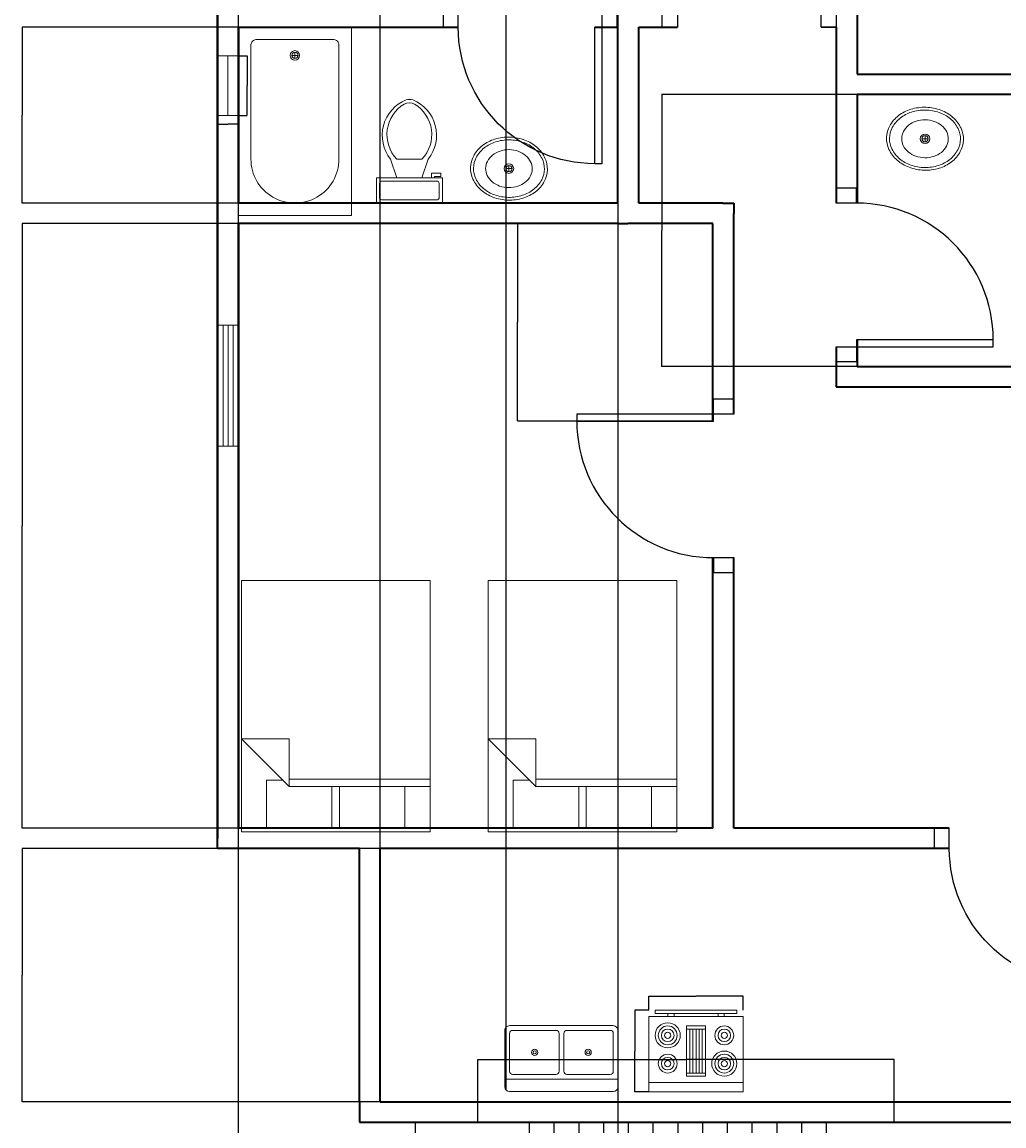
# Model space of a CAD drawing. Units: millimetres. Extents: x 31 to 27050, y -916 to 32407.
# Tile 5 of 7: x 31 to 7965, y 16782 to 25704. Entities that reach past the tile are written whole.
import ezdxf

# ---------------------------------------------------------------- set-up
doc = ezdxf.new("R2010")
doc.units = ezdxf.units.MM
for name, color, linetype, lineweight in [('A-ANNO-DIMS', 2, 'Continuous', 18), ('A-DOOR', 3, 'Continuous', 25), ('A-EQPM', 8, 'Continuous', 18), ('A-FLOR-FIXT', 9, 'Continuous', 18), ('A-FLOR-STRS', 7, 'Continuous', 25), ('A-FURN', 8, 'Continuous', 13), ('A-GLAZ', 4, 'Continuous', 18), ('A-WALL', 7, 'Continuous', 35)]:
    doc.layers.add(name, color=color, linetype=linetype, lineweight=lineweight)
doc.styles.get("Standard").update_dxf_attribs({"font": 'arial.ttf'})
doc.dimstyles.get("Standard").update_dxf_attribs({"dimtxt": 0.18, "dimasz": 0.18, "dimexe": 0.18, "dimexo": 0.0625, "dimgap": 0.09, "dimtad": 0, "dimtih": 1, "dimtoh": 1, "dimdec": 4, "dimzin": 0, "dimdsep": 46, "dimtxsty": 'Standard', "dimcen": 0.09, "dimadec": 0, "dimazin": 0, "dimtfac": 1, "dimtdec": 4, "dimtofl": 0, "dimtmove": 0, "dimatfit": 3, "dimfxl": 1, "dimtolj": 1, "dimtzin": 0, "dimarcsym": 0})

# ---------------------------------------------------------------- blocks, each defined once
blk = doc.blocks.new('Range-Oven - 30 in top')
for p, q in [((0, -3), (30, -3)), ((12, -6), (18, -6)), ((13, -19.999996), (13, -6)), ((14, -6), (14, -19.999996)), ((15, -19.999996), (15, -6)), ((16, -6), (16, -19.999996)), ((17, -19.999996), (17, -6)), ((18, -19.999996), (12, -19.999996)), ((6.000000000000003, -23.99999600000001), (6.000000000000003, -24.999996)), ((8.000000000000004, -24.999996), (8.000000000000004, -23.99999600000001)), ((22.00000000000001, -24.999996), (22.00000000000001, -23.99999600000001)), ((24, -23.99999600000001), (24, -24.999996))]:
    blk.add_line(p, q)
for points in [[(0, -23.99999600000001), (0, 0), (30, 0), (30, -23.99999600000001)], [(12, -20.999996), (12, -5), (18, -5), (18, -20.999996)], [(2.000000000000003, -25.999996), (2.000000000000003, -24.999996), (28.00000000000001, -24.999996), (28.00000000000001, -25.999996)]]:
    blk.add_lwpolyline(points, close=True)
for centre, radius in [((6.000000000000003, -9.0000002), 4), ((6.000000000000003, -9.0000002), 3), ((6.000000000000003, -9.0000002), 2), ((24, -9.0000002), 3), ((24, -9.0000002), 2), ((6.000000000000003, -9.0000002), 1), ((24, -9.0000002), 1), ((24, -18), 4), ((6.000000000000003, -18), 3), ((6.000000000000003, -18), 2), ((6.000000000000003, -18), 1), ((24, -18), 3), ((24, -18), 2), ((24, -18), 1)]:
    blk.add_circle(centre, radius)
blk = doc.blocks.new('Sink-double - 36 in top')
for p, q in [((-18, -4), (18, -4)), ((-0.75, -18.5), (-0.75, -6.5)), ((0.75, -6.5), (0.75, -18.5))]:
    blk.add_line(p, q)
for points in [[(-16.5, 0), (16.5, 0)], [(-18, -19.5), (-18, -1.5)], [(18, -1.5), (18, -19.5)], [(-16.5, -18.5), (-16.5, -6.5)], [(-15.5, -5.5), (-1.75, -5.5)], [(1.75, -5.5), (15.5, -5.5)], [(16.5, -6.5), (16.5, -18.5)], [(16.5, -21), (-16.5, -21)], [(-1.75, -19.5), (-15.5, -19.5)], [(15.5, -19.5), (1.75, -19.5)]]:
    blk.add_lwpolyline(points)
for centre, radius in [((-8.5, -12.5), 1), ((-8.5, -12.5), 0.5), ((8.5, -12.5), 1), ((8.5, -12.5), 0.5)]:
    blk.add_circle(centre, radius)
for centre, radius, start, end in [((-16.5, -1.5), 1.5, 90, 180), ((16.5, -1.5), 1.5, 0, 90), ((-15.5, -6.5), 1, 90, 180), ((-1.75, -6.5), 1, 0, 90), ((1.75, -6.5), 1, 90, 180), ((15.5, -6.5), 1, 0, 90), ((-16.5, -19.5), 1.5, 180, 270), ((-15.5, -18.5), 1, 180, 270), ((-1.75, -18.5), 1, 270, 0), ((1.75, -18.5), 1, 180, 270), ((15.5, -18.5), 1, 270, 0), ((16.5, -19.5), 1.5, 270, 0)]:
    blk.add_arc(centre, radius, start, end)
blk = doc.blocks.new('Bath Tub - 26 x 60 in.')
for p, q in [((9, -17), (9, -19)), ((8, -18), (10, -18))]:
    blk.add_line(p, q)
blk.add_lwpolyline([(0, -36), (0, 0), (60, 0), (60, -36)], close=True)
for points in [[(4, -30), (4, -6)], [(6, -4), (42, -4)], [(42, -32), (6, -32)]]:
    blk.add_lwpolyline(points)
for radius in [1.5, 1]:
    blk.add_circle((9, -18), radius)
for centre, radius, start, end in [((5.75, -5.75), 1.767766999999999, 81.86989999999999, 188.1301), ((42, -18), 14, 270, 90), ((5.75, -30.25), 1.767766999999999, 171.8699, 278.1301)]:
    blk.add_arc(centre, radius, start, end)
blk = doc.blocks.new('Sink - Oval top')
for p, q in [((-1, 0), (1, 0)), ((0, 1), (0, -1))]:
    blk.add_line(p, q)
for points in [[(-12.23371880354079, 0.3941914712607968, 0.1176342565883263), (-11.46456229543957, -3.361933235489118, 0.104469279667093), (-8.878748691070427, -6.803541973650567, 0.0900157896014849), (-5.082757700676665, -9.072309807490512, 0.0819199491592185), (-0.3227280122732736, -10.01585280257211, 0.0819199491592091), (4.488169920880977, -9.380701564817912, 0.0900157896014801), (8.422342359155778, -7.36101289847943, 0.1044692796670922), (11.22435122606941, -4.093009071543406, 0.1176342565883338), (12.23371880354091, -0.3941914712607968, 0.1176342565883057), (11.46456229543992, 3.361933235488777, 0.1044692796670849), (8.878748691070427, 6.803541973650567, 0.0900157896014884), (5.082757700676324, 9.072309807490681, 0.0819199491592058), (0.3227280122732736, 10.01585280257211, 0.081919949159207), (-4.488169920880864, 9.380701564817969, 0.0900157896014802), (-8.422342359155778, 7.36101289847943, 0.1044692796670951), (-11.22435122606919, 4.093009071543633, 0.1176342565883402)], [(-11.28627986850119, 0.1590597164737346, 0.1186217001864142), (-10.51590095791209, -3.253161772358112, 0.1046781721811095), (-8.071803350560115, -6.358618019863342, 0.0895620664691738), (-4.537699193222351, -8.366971929609804, 0.0811846988912177), (-0.1289739026695997, -9.15150355811437, 0.0811846988912276), (4.300109150126218, -8.491524865184601, 0.0895620664691798), (7.889406708212618, -6.583562428127606, 0.1046781721811044), (10.42004782883111, -3.548216131892445, 0.1186217001864013), (11.28627986850119, -0.1590597164736209, 0.1186217001863945), (10.51590095791221, 3.253161772357998, 0.1046781721811069), (8.071803350560115, 6.358618019863342, 0.0895620664691756), (4.537699193222124, 8.366971929609917, 0.081184698891216), (0.1289739026695997, 9.151503558114428, 0.0811846988912142), (-4.300109150125877, 8.491524865184829, 0.0895620664691747), (-7.889406708212618, 6.583562428127606, 0.1046781721811045), (-10.42004782883111, 3.548216131892445, 0.1186217001863946)], [(-7.420452389032902, 0.0829876781601797, 0.1182825673856775), (-6.907065465214486, -2.1674649380775, 0.1046074595377274), (-5.294791470712084, -4.209988192029413, 0.0897179636260996), (-2.966599981142508, -5.528122152688069, 0.0814360825277113), (-0.0675135187855176, -6.036810076758797, 0.0814360825277218), (2.84222437824053, -5.593085960977873, 0.0897179636261315), (5.199312936802016, -4.327350491993342, 0.1046074595376878), (6.85686365682659, -2.321395784920355, 0.1182825673856714), (7.420452389033016, -0.0829876781601797, 0.1182825673856961), (6.907065465214486, 2.167464938077614, 0.1046074595377135), (5.294791470712084, 4.209988192029413, 0.0897179636261265), (2.966599981142621, 5.528122152687842, 0.0814360825277426), (0.0675135187855176, 6.036810076758797, 0.0814360825277225), (-2.842224378240644, 5.593085960977873, 0.0897179636261212), (-5.199312936802016, 4.327350491993342, 0.1046074595377049), (-6.856863656826476, 2.321395784920355, 0.1182825673856712)]]:
    blk.add_lwpolyline(points, format="xyb", close=True)
for radius in [1.5, 1]:
    blk.add_circle((0, 0), radius)
blk = doc.blocks.new('Toilet - top')
for p, q in [((9.5, -6), (9.5, -2)), ((-10, -8.5), (-8, -8.5)), ((-10, -9.5), (-10, -8.5)), ((-7, -9.5), (-10, -9.5)), ((-8, -8.5), (-8, -8)), ((-7, -8), (-7, -9.5)), ((-4, -8), (-6, -14)), ((4, -8), (6, -14)), ((4, -14), (-4, -14))]:
    blk.add_line(p, q)
blk.add_lwpolyline([(10.5, -8), (10.5, 0), (-10.5, 0), (-10.5, -8)], close=True)
for points in [[(-9.5, -2), (-9.5, -6)], [(8.5, -1), (-8.5, -1)], [(-8.5, -7), (8.5, -7)]]:
    blk.add_lwpolyline(points)
for centre, radius, start, end in [((-8.625, -1.875), 0.8838834999999999, 81.86989999999999, 188.1301), ((8.625, -1.875), 0.8838834999999999, 351.8699, 98.13009999999998), ((-8.625, -6.125), 0.8838834999999999, 171.869898, 278.1301), ((8.625, -6.125), 0.8838834999999999, 261.8699, 8.130099999999993), ((3.519562435188956, -21.58049502388982), 12.16902005083646, 141.4691096810948, 247.9714346835576), ((4.199957580658807, -21.81740929088453), 11.3291791325804, 136.3677254423718, 238.946823937405), ((-3.519499936778316, -21.58047137067522), 12.16903423757823, 292.0284332733152, 38.53070636800453), ((-4.199890672038477, -21.81738596564128), 11.32918622148567, 301.0530065773863, 43.63209216694732), ((2.09660981727e-05, -27.87646475467881), 4, 245.7318247449371, 294.2681740488959), ((2.09415214183e-05, -28.99996806116075), 4, 254.8605283244437, 285.1394707718433)]:
    blk.add_arc(centre, radius, start, end)
blk = doc.blocks.new('Bed - Queen')
for p, q in [((0, -80.00003000000002), (0, 0)), ((0, 0), (59.99998999999999, 0)), ((59.99998999999999, 0), (59.99998999999999, -80.00003000000002)), ((7.99999, -1.200000000000017), (28.79998, -1.200000000000017)), ((7.99999, -14.4), (7.99999, -1.200000000000017)), ((28.79998, -1.200000000000017), (28.79998, -14.4)), ((31.19999, -1.200000000000017), (51.99999000000001, -1.200000000000017)), ((31.19999, -14.4), (31.19999, -1.200000000000017)), ((51.99999000000001, -1.200000000000017), (51.99999000000001, -16.4)), ((0, -14.4), (44.79999999999999, -14.4)), ((44.79999999999999, -16.80000000000001), (0, -16.80000000000001)), ((59.99998999999999, -29.60000000000001), (44.79999999999999, -14.4)), ((44.79999999999999, -14.4), (44.79999999999999, -29.60000000000001)), ((51.99999000000001, -16.4), (46.79936, -16.4)), ((44.79999999999999, -29.60000000000001), (59.99998999999999, -29.60000000000001)), ((59.99998999999999, -80.00003000000002), (0, -80.00003000000002))]:
    blk.add_line(p, q)
blk = doc.blocks.new('Window - Wood Frame 36 in. Wide plan')
for p, q in [((0, 6), (0, 0)), ((0, 4.5), (36, 4.5)), ((36, 6), (36, 0)), ((0, 3), (36, 3)), ((0, 1.5), (36, 1.5))]:
    blk.add_line(p, q)
blk = doc.blocks.new('DOOR-SINGLE-1104')
for p, q in [((56.41678681898429, 1104.337341461596), (-7.18501e-11, 1104.337341461596)), ((-7.18501e-11, 1104.337341461596), (-7.18501e-11, 3.638e-12)), ((56.41678681898429, 7.276e-12), (56.41678681898429, 1104.337341461596)), ((-1226.913698425656, -163.8831223050438), (-1226.913698425656, 3.638e-12)), ((-1104.337341461589, 3.638e-12), (-1226.913698425656, 7.276e-12)), ((-1104.337341461589, 3.638e-12), (-1104.337341461589, -163.8831223050438)), ((-7.18501e-11, 3.638e-12), (56.41678681898429, 7.276e-12)), ((56.41678681898429, -163.8831223050438), (56.41678681898429, 3.638e-12)), ((56.41678681898429, 3.638e-12), (178.9931437830519, 3.638e-12)), ((178.9931437830519, 3.638e-12), (178.9931437830519, -163.8831223050438)), ((-1104.337341461589, -163.8831223050438), (-1226.913698425656, -163.8831223050438)), ((178.9931437830519, -163.8831223050438), (56.41678681898429, -163.8831223050438))]:
    blk.add_line(p, q)
blk.add_arc((0, 3.638e-12), 1104.337341461589, 90, 180)
blk = doc.blocks.new('STAIR-RETURN-2400')
for p, q in [((9.095e-13, 2345.636859649549), (9.095e-13, -1.819e-12)), ((200.0000000000009, 2345.636859649549), (200.0000000000009, -1.819e-12)), ((400.0000000000008, 2345.636859649549), (400.0000000000008, -1.819e-12)), ((600.0000000000008, 2345.636859649549), (600.0000000000008, -1.819e-12)), ((800.0000000000008, 2345.636859649552), (800.0000000000008, 1.819e-12)), ((1000.000000000001, 2345.636859649556), (1000.000000000001, 5.457e-12)), ((1200.000000000001, 2345.636859649556), (1200.000000000001, 5.457e-12)), ((1400.000000000001, 2345.636859649556), (1400.000000000001, 5.457e-12)), ((1600.000000000001, 2345.636859649559), (1600.000000000001, 9.0949e-12)), ((1800.000000000001, 2345.636859649559), (1800.000000000001, 9.0949e-12)), ((2000.000000000001, 2345.636859649559), (2000.000000000001, 9.0949e-12)), ((2200.000000000001, 2345.636859649563), (2200.000000000001, 1.27329e-11)), ((2400.000000000001, 2345.636859649563), (2400.000000000001, 1.27329e-11)), ((-415.9249645337103, 697.4958917418807), (-415.9249645337103, 1817.654410237617)), ((-415.9249645337103, 1817.654410237617), (2588.331988211024, 1817.654410237617)), ((9.095e-13, 1172.818429824772), (9.095e-13, 1272.818429824772)), ((9.095e-13, 1272.818429824772), (2400.000000000001, 1272.818429824774)), ((2400.000000000001, 1272.818429824774), (2400.000000000001, 1072.818429824774)), ((2400.000000000001, 1072.818429824774), (9.095e-13, 1072.818429824774)), ((2597.09055342863, 697.4958917418807), (-415.9249645337103, 697.4958917418807))]:
    blk.add_line(p, q)
blk.add_lwpolyline([(2948.607295106225, 1817.654410237617), (2588.331988211024, 2025.65945565594), (2588.331988211024, 1609.649364819299)], close=True)
blk = doc.blocks.new('WIN-BATH-482')
for p, q in [((0, 3.638e-12), (-168.350650710694, 3.638e-12)), ((-84.17532535534633, -482.3297634273148), (-84.17532535534701, 3.638e-12)), ((-168.350650710694, -482.3297634273148), (1.3642e-12, -482.3297634273148))]:
    blk.add_line(p, q)
blk = doc.blocks.new('*D30')
at = {"layer": 'A-ANNO-DIMS', "color": 0, "lineweight": -2, "transparency": 16777216}
for p, q in [((5095.835211668338, 17717.30289499948), (5095.835211668338, 17831.72039499948)), ((5096.015211668339, 17831.54039499948), (5475.759816033958, 17831.54039499948)), ((5857.655211668338, 17831.54039499948), (5477.910607302717, 17831.54039499948)), ((5857.835211668338, 17717.30289499948), (5857.835211668338, 17831.72039499948))]:
    blk.add_line(p, q, dxfattribs=at)
at = {"layer": 'A-ANNO-DIMS', "color": 0, "transparency": 16777216}
for points in [[(5096.015211668339, 17831.57039499948), (5096.015211668339, 17831.51039499948), (5095.835211668338, 17831.54039499948)], [(5857.655211668338, 17831.57039499948), (5857.655211668338, 17831.51039499948), (5857.835211668338, 17831.54039499948)]]:
    blk.add_solid(points, dxfattribs=at)
at = {"layer": 'Defpoints', "color": 0, "transparency": 16777216}
for p in [(5095.835211668338, 17831.54039499948), (5095.835211668338, 17717.24039499948), (5857.835211668338, 17717.24039499948)]:
    blk.add_point(p, dxfattribs=at)
at = {"layer": 'A-ANNO-DIMS', "color": 0, "transparency": 16777216, "insert": (5476.835211668338, 17831.54039499948), "char_height": 0.18, "attachment_point": 5}
blk.add_mtext('\\A1;RANGE 762 TYP.', dxfattribs=at)
blk = doc.blocks.new('*D31')
at = {"layer": 'A-ANNO-DIMS', "color": 0, "lineweight": -2, "transparency": 16777216}
for p, q in [((5095.77271166834, 17717.24039499949), (4981.355211668341, 17717.24039499949)), ((4981.535211668341, 17717.06039499949), (4981.535211668341, 17387.22234893728)), ((4981.535211668341, 17057.02049659949), (4981.535211668341, 17386.8585426617)), ((5095.77271166834, 17056.84049659949), (4981.355211668341, 17056.84049659949))]:
    blk.add_line(p, q, dxfattribs=at)
at = {"layer": 'A-ANNO-DIMS', "color": 0, "transparency": 16777216}
for points in [[(4981.505211668341, 17717.06039499949), (4981.565211668342, 17717.06039499949), (4981.535211668341, 17717.24039499949)], [(4981.505211668341, 17057.02049659949), (4981.565211668342, 17057.02049659949), (4981.535211668341, 17056.84049659949)]]:
    blk.add_solid(points, dxfattribs=at)
at = {"layer": 'Defpoints', "color": 0, "transparency": 16777216}
for p in [(5095.83521166834, 17717.24039499949), (4981.535211668341, 17056.84049659949), (5095.83521166834, 17056.84049659949)]:
    blk.add_point(p, dxfattribs=at)
at = {"layer": 'A-ANNO-DIMS', "color": 0, "transparency": 16777216, "insert": (4981.535211668346, 17387.04044579948), "char_height": 0.18, "attachment_point": 5}
blk.add_mtext('\\A1;660 TYP.', dxfattribs=at)
blk = doc.blocks.new('*D40')
at = {"layer": 'A-ANNO-DIMS', "color": 0, "lineweight": -2, "transparency": 16777216}
for p, q in [((3712.669091999182, 16813.12429635636), (3712.669091999182, 17317.92163530235)), ((3712.849091999181, 17317.74163530235), (5393.307977617239, 17317.74163530235)), ((7077.021351639117, 17317.74163530235), (5396.562466021059, 17317.74163530235)), ((7077.201351639117, 16813.12429635636), (7077.201351639117, 17317.92163530235))]:
    blk.add_line(p, q, dxfattribs=at)
at = {"layer": 'A-ANNO-DIMS', "color": 0, "transparency": 16777216}
for points in [[(3712.849091999181, 17317.77163530235), (3712.849091999181, 17317.71163530235), (3712.669091999182, 17317.74163530235)], [(7077.021351639117, 17317.77163530235), (7077.021351639117, 17317.71163530235), (7077.201351639117, 17317.74163530235)]]:
    blk.add_solid(points, dxfattribs=at)
at = {"layer": 'Defpoints', "color": 0, "transparency": 16777216}
for p in [(7077.201351639117, 17317.74163530235), (3712.669091999182, 16813.06179635636), (7077.201351639117, 16813.06179635636)]:
    blk.add_point(p, dxfattribs=at)
at = {"layer": 'A-ANNO-DIMS', "color": 0, "transparency": 16777216, "insert": (5394.935221819149, 17317.74163530235), "char_height": 0.18, "attachment_point": 5}
blk.add_mtext('\\A1;RETURN STAIR 3365 TYP.', dxfattribs=at)
blk = doc.blocks.new('*D41')
at = {"layer": 'A-ANNO-DIMS', "color": 0, "lineweight": -2, "transparency": 16777216}
for p, q in [((3712.606591999184, 16813.06179635637), (3207.809253053195, 16813.06179635637)), ((3207.989253053195, 16812.88179635637), (3207.989253053195, 15640.42533106092)), ((3207.989253053195, 14467.60493670681), (3207.989253053195, 15640.06140200226)), ((3712.606591999184, 14467.4249367068), (3207.809253053195, 14467.4249367068))]:
    blk.add_line(p, q, dxfattribs=at)
at = {"layer": 'A-ANNO-DIMS', "color": 0, "transparency": 16777216}
for points in [[(3207.959253053195, 16812.88179635637), (3208.019253053195, 16812.88179635637), (3207.989253053195, 16813.06179635637)], [(3207.959253053195, 14467.60493670681), (3208.019253053195, 14467.60493670681), (3207.989253053195, 14467.4249367068)]]:
    blk.add_solid(points, dxfattribs=at)
at = {"layer": 'Defpoints', "color": 0, "transparency": 16777216}
for p in [(3207.989253053195, 16813.06179635637), (3712.669091999184, 16813.06179635637), (3712.669091999184, 14467.4249367068)]:
    blk.add_point(p, dxfattribs=at)
at = {"layer": 'A-ANNO-DIMS', "color": 0, "transparency": 16777216, "insert": (3207.989253053199, 15640.24336653158), "char_height": 0.18, "attachment_point": 5}
blk.add_mtext('\\A1;2346 TYP.', dxfattribs=at)
blk = doc.blocks.new('*D44')
at = {"layer": 'A-ANNO-DIMS', "color": 0, "lineweight": -2, "transparency": 16777216}
for p, q in [((1778.435147825163, 25432.43652884754), (1850.902112339262, 25432.43652884754)), ((1850.722112339262, 25432.25652884754), (1850.722112339262, 25191.4547781025)), ((1850.722112339262, 24950.28676542022), (1850.722112339262, 25191.08851616526)), ((1778.435147825163, 24950.10676542022), (1850.902112339262, 24950.10676542022))]:
    blk.add_line(p, q, dxfattribs=at)
at = {"layer": 'A-ANNO-DIMS', "color": 0, "transparency": 16777216}
for points in [[(1850.692112339262, 25432.25652884754), (1850.752112339262, 25432.25652884754), (1850.722112339262, 25432.43652884754)], [(1850.692112339262, 24950.28676542022), (1850.752112339262, 24950.28676542022), (1850.722112339262, 24950.10676542022)]]:
    blk.add_solid(points, dxfattribs=at)
at = {"layer": 'Defpoints', "color": 0, "transparency": 16777216}
for p in [(1778.372647825163, 25432.43652884754), (1850.722112339262, 25432.43652884754), (1778.372647825163, 24950.10676542022)]:
    blk.add_point(p, dxfattribs=at)
at = {"layer": 'A-ANNO-DIMS', "color": 0, "transparency": 16777216, "insert": (1850.722112339269, 25191.27164713387), "char_height": 0.18, "attachment_point": 5}
blk.add_mtext('\\A1;BATH WINDOW 482 TYP.', dxfattribs=at)
blk = doc.blocks.new('*D45')
at = {"layer": 'A-ANNO-DIMS', "color": 0, "lineweight": -2, "transparency": 16777216}
for p, q in [((1610.021997114467, 24950.04426542021), (1610.021997114467, 24877.57730090611)), ((1778.372647825162, 24950.04426542021), (1778.372647825162, 24877.57730090611)), ((1610.201997114467, 24877.75730090611), (1693.607779495735, 24877.75730090611)), ((1778.192647825162, 24877.75730090611), (1694.786865443894, 24877.75730090611))]:
    blk.add_line(p, q, dxfattribs=at)
at = {"layer": 'A-ANNO-DIMS', "color": 0, "transparency": 16777216}
for points in [[(1610.201997114467, 24877.78730090611), (1610.201997114467, 24877.72730090611), (1610.021997114467, 24877.75730090611)], [(1778.192647825162, 24877.78730090611), (1778.192647825162, 24877.72730090611), (1778.372647825162, 24877.75730090611)]]:
    blk.add_solid(points, dxfattribs=at)
at = {"layer": 'Defpoints', "color": 0, "transparency": 16777216}
for p in [(1610.021997114467, 24950.10676542021), (1778.372647825162, 24950.10676542021), (1778.372647825162, 24877.75730090611)]:
    blk.add_point(p, dxfattribs=at)
at = {"layer": 'A-ANNO-DIMS', "color": 0, "transparency": 16777216, "insert": (1694.197322469815, 24877.75730090611), "char_height": 0.18, "attachment_point": 5}
blk.add_mtext('\\A1;168 TYP.', dxfattribs=at)
blk = doc.blocks.new('*D53')
at = {"layer": 'A-ANNO-DIMS', "color": 0, "lineweight": -2, "transparency": 16777216}
for p, q in [((1778.310148000001, 25663.64813600002), (30.84199699999976, 25663.64813600002)), ((31.02199699999987, 25663.46813600001), (31.02199700000003, 24952.32387752935)), ((31.02199700000019, 24240.81569000001), (31.02199700000003, 24951.95994847068)), ((1778.310148000001, 24240.63569000001), (30.84199700000008, 24240.63569000001))]:
    blk.add_line(p, q, dxfattribs=at)
at = {"layer": 'A-ANNO-DIMS', "color": 0, "transparency": 16777216}
for points in [[(30.99199699999987, 25663.46813600001), (31.05199699999988, 25663.46813600001), (31.02199699999987, 25663.64813600002)], [(30.99199700000019, 24240.81569000001), (31.05199700000019, 24240.81569000001), (31.02199700000019, 24240.63569000001)]]:
    blk.add_solid(points, dxfattribs=at)
at = {"layer": 'Defpoints', "color": 0, "transparency": 16777216}
for p in [(31.02199699999987, 25663.64813600002), (1778.372648000001, 25663.64813600002), (1778.372648000001, 24240.63569000001)]:
    blk.add_point(p, dxfattribs=at)
at = {"layer": 'A-ANNO-DIMS', "color": 0, "transparency": 16777216, "insert": (31.02199700000709, 24952.14191300001), "char_height": 0.18, "attachment_point": 5}
blk.add_mtext('\\A1;1423', dxfattribs=at)
blk = doc.blocks.new('*D54')
at = {"layer": 'A-ANNO-DIMS', "color": 0, "lineweight": -2, "transparency": 16777216}
for p, q in [((1778.310148000001, 24076.75256800001), (30.84199699999943, 24076.75256800001)), ((31.02199699999948, 24076.57256800001), (31.02199700000003, 21633.2176101378)), ((31.02199700000057, 19189.498846), (31.02199700000003, 21632.85380386222)), ((1778.310148000001, 19189.318846), (30.84199700000052, 19189.318846))]:
    blk.add_line(p, q, dxfattribs=at)
at = {"layer": 'A-ANNO-DIMS', "color": 0, "transparency": 16777216}
for points in [[(30.99199699999948, 24076.57256800001), (31.05199699999948, 24076.57256800001), (31.02199699999948, 24076.75256800001)], [(30.99199700000057, 19189.498846), (31.05199700000057, 19189.498846), (31.02199700000057, 19189.318846)]]:
    blk.add_solid(points, dxfattribs=at)
at = {"layer": 'Defpoints', "color": 0, "transparency": 16777216}
for p in [(31.02199699999948, 24076.75256800001), (1778.372648000001, 24076.75256800001), (1778.372648000001, 19189.318846)]:
    blk.add_point(p, dxfattribs=at)
at = {"layer": 'A-ANNO-DIMS', "color": 0, "transparency": 16777216, "insert": (31.02199700000615, 21633.03570700001), "char_height": 0.18, "attachment_point": 5}
blk.add_mtext('\\A1;4887', dxfattribs=at)
blk = doc.blocks.new('*D55')
at = {"layer": 'A-ANNO-DIMS', "color": 0, "lineweight": -2, "transparency": 16777216}
for p, q in [((2925.628986000001, 19025.43572400001), (30.84199699999987, 19025.43572400001)), ((31.0219969999998, 19025.255724), (31.02199700000003, 18001.3722246378)), ((31.02199700000026, 16977.12491900001), (31.02199700000003, 18001.00841836222)), ((2925.628986000001, 16976.94491900001), (30.84199700000032, 16976.94491900001))]:
    blk.add_line(p, q, dxfattribs=at)
at = {"layer": 'A-ANNO-DIMS', "color": 0, "transparency": 16777216}
for points in [[(30.9919969999998, 19025.255724), (31.0519969999998, 19025.255724), (31.0219969999998, 19025.43572400001)], [(30.99199700000025, 16977.12491900001), (31.05199700000026, 16977.12491900001), (31.02199700000026, 16976.94491900001)]]:
    blk.add_solid(points, dxfattribs=at)
at = {"layer": 'Defpoints', "color": 0, "transparency": 16777216}
for p in [(31.0219969999998, 19025.43572400001), (2925.691486000001, 19025.43572400001), (2925.691486000001, 16976.94491900001)]:
    blk.add_point(p, dxfattribs=at)
at = {"layer": 'A-ANNO-DIMS', "color": 0, "transparency": 16777216, "insert": (31.02199700000512, 18001.1903215), "char_height": 0.18, "attachment_point": 5}
blk.add_mtext('\\A1;2048.5', dxfattribs=at)
blk = doc.blocks.new('*D61')
at = {"layer": 'A-ANNO-DIMS', "color": 0, "lineweight": -2, "transparency": 16777216}
for p, q in [((1778.372648, 7250.606205), (1778.372648000001, 32406.711259)), ((1778.552648000001, 32406.531259), (3312.109331318556, 32406.531259)), ((4846.592413000001, 32406.531259), (3313.035729681448, 32406.531259)), ((4846.772413, 7250.606205), (4846.772413000001, 32406.711259))]:
    blk.add_line(p, q, dxfattribs=at)
at = {"layer": 'A-ANNO-DIMS', "color": 0, "transparency": 16777216}
for points in [[(1778.552648000001, 32406.561259), (1778.552648000001, 32406.501259), (1778.372648000001, 32406.531259)], [(4846.592413000001, 32406.561259), (4846.592413000001, 32406.501259), (4846.772413000001, 32406.531259)]]:
    blk.add_solid(points, dxfattribs=at)
at = {"layer": 'Defpoints', "color": 0, "transparency": 16777216}
for p in [(4846.772413000001, 32406.531259), (1778.372648, 7250.543705), (4846.772413, 7250.543705)]:
    blk.add_point(p, dxfattribs=at)
at = {"layer": 'A-ANNO-DIMS', "color": 0, "transparency": 16777216, "insert": (3312.572530500002, 32406.531259), "char_height": 0.18, "attachment_point": 5}
blk.add_mtext('\\A1;3068.4', dxfattribs=at)
blk = doc.blocks.new('*D62')
at = {"layer": 'A-ANNO-DIMS', "color": 0, "lineweight": -2, "transparency": 16777216}
for p, q in [((6778.310148000002, 25117.33256500002), (5199.192648000003, 25117.33256500002)), ((5199.372648000004, 25117.15256500002), (5199.372648000004, 24018.8323336378)), ((5199.372648000004, 22920.14829600001), (5199.372648000004, 24018.46852736222)), ((6778.310148000002, 22919.96829600001), (5199.192648000003, 22919.96829600001))]:
    blk.add_line(p, q, dxfattribs=at)
at = {"layer": 'A-ANNO-DIMS', "color": 0, "transparency": 16777216}
for points in [[(5199.342648000004, 25117.15256500002), (5199.402648000003, 25117.15256500002), (5199.372648000004, 25117.33256500002)], [(5199.342648000004, 22920.14829600001), (5199.402648000003, 22920.14829600001), (5199.372648000004, 22919.96829600001)]]:
    blk.add_solid(points, dxfattribs=at)
at = {"layer": 'Defpoints', "color": 0, "transparency": 16777216}
for p in [(5199.372648000004, 25117.33256500002), (6778.372648000003, 25117.33256500002), (6778.372648000003, 22919.96829600001)]:
    blk.add_point(p, dxfattribs=at)
at = {"layer": 'A-ANNO-DIMS', "color": 0, "transparency": 16777216, "insert": (5199.37264800001, 24018.65043050001), "char_height": 0.18, "attachment_point": 5}
blk.add_mtext('\\A1;2197.4', dxfattribs=at)
blk = doc.blocks.new('*D66')
at = {"layer": 'A-ANNO-DIMS', "color": 0, "lineweight": -2, "transparency": 16777216}
for p, q in [((2925.691486, 19025.498224), (2925.691486000001, 32406.711259)), ((2925.871486000001, 32406.531259), (6219.151999023875, 32406.531259)), ((9513.151407, 32406.531259), (6219.870893976127, 32406.531259)), ((9513.331407, 19025.498224), (9513.331407, 32406.711259))]:
    blk.add_line(p, q, dxfattribs=at)
at = {"layer": 'A-ANNO-DIMS', "color": 0, "transparency": 16777216}
for points in [[(2925.871486000001, 32406.561259), (2925.871486000001, 32406.501259), (2925.691486000001, 32406.531259)], [(9513.151407, 32406.561259), (9513.151407, 32406.501259), (9513.331407, 32406.531259)]]:
    blk.add_solid(points, dxfattribs=at)
at = {"layer": 'Defpoints', "color": 0, "transparency": 16777216}
for p in [(9513.331407, 32406.531259), (2925.691486, 19025.435724), (9513.331407, 19025.435724)]:
    blk.add_point(p, dxfattribs=at)
at = {"layer": 'A-ANNO-DIMS', "color": 0, "transparency": 16777216, "insert": (6219.511446500001, 32406.531259), "char_height": 0.18, "attachment_point": 5}
blk.add_mtext('\\A1;6588', dxfattribs=at)
blk = doc.blocks.new('*D90')
at = {"layer": 'A-ANNO-DIMS', "color": 0, "lineweight": -2, "transparency": 16777216}
for p, q in [((5613.294525000002, 24076.75256800001), (4034.177025000002, 24076.75256800001)), ((4034.357025000002, 24076.57256800001), (4034.357025000003, 23278.30521152934)), ((4034.357025000003, 22479.67392600001), (4034.357025000003, 23277.94128247067)), ((5613.294525000002, 22479.49392600001), (4034.177025000003, 22479.49392600001))]:
    blk.add_line(p, q, dxfattribs=at)
at = {"layer": 'A-ANNO-DIMS', "color": 0, "transparency": 16777216}
for points in [[(4034.327025000003, 24076.57256800001), (4034.387025000003, 24076.57256800001), (4034.357025000002, 24076.75256800001)], [(4034.327025000003, 22479.67392600001), (4034.387025000003, 22479.67392600001), (4034.357025000003, 22479.49392600001)]]:
    blk.add_solid(points, dxfattribs=at)
at = {"layer": 'Defpoints', "color": 0, "transparency": 16777216}
for p in [(4034.357025000002, 24076.75256800001), (5613.357025000002, 24076.75256800001), (5613.357025000002, 22479.49392600001)]:
    blk.add_point(p, dxfattribs=at)
at = {"layer": 'A-ANNO-DIMS', "color": 0, "transparency": 16777216, "insert": (4034.357025000009, 23278.123247), "char_height": 0.18, "attachment_point": 5}
blk.add_mtext('\\A1;1597.3', dxfattribs=at)
blk = doc.blocks.new('*D94')
at = {"layer": 'A-ANNO-DIMS', "color": 0, "lineweight": -2, "transparency": 16777216}
for p, q in [((2925.691486, 16977.007419), (2925.691486000001, 32406.711259)), ((2925.871486000001, 32406.531259), (3434.121002435881, 32406.531259)), ((3943.281201000001, 32406.531259), (3435.031684564121, 32406.531259)), ((3943.461201, 17070.178763), (3943.461201000001, 32406.711259))]:
    blk.add_line(p, q, dxfattribs=at)
at = {"layer": 'A-ANNO-DIMS', "color": 0, "transparency": 16777216}
for points in [[(2925.871486000001, 32406.561259), (2925.871486000001, 32406.501259), (2925.691486000001, 32406.531259)], [(3943.281201000001, 32406.561259), (3943.281201000001, 32406.501259), (3943.461201000001, 32406.531259)]]:
    blk.add_solid(points, dxfattribs=at)
at = {"layer": 'Defpoints', "color": 0, "transparency": 16777216}
for p in [(3943.461201000001, 32406.531259), (3943.461201, 17070.116263), (2925.691486, 16976.944919)]:
    blk.add_point(p, dxfattribs=at)
at = {"layer": 'A-ANNO-DIMS', "color": 0, "transparency": 16777216, "insert": (3434.576343500001, 32406.531259), "char_height": 0.18, "attachment_point": 5}
blk.add_mtext('\\A1;1017.8', dxfattribs=at)

msp = doc.modelspace()

# ---------------------------------------------------------------- linework, layer by layer
at = {"layer": 'A-DOOR'}
msp.add_line((6487.445640150401, 25663.64813636669), (6610.021997114468, 25663.64813636669), dxfattribs=at)
at = {"layer": 'A-WALL'}
for p, q in [((1610.021997114467, 30744.38037777559), (1610.021997114467, 19106.16796530105)), ((1610.021997114469, 19025.43572389214), (1610.021997114469, 30744.3803777756)), ((6778.372647825161, 30663.64813636668), (6778.372647825161, 25282.64192458121)), ((1778.372647825163, 25663.64813636668), (3555.456298411929, 25663.64813636669)), ((1778.372647825161, 25663.64813636668), (1778.372647825161, 24240.63568990879)), ((1778.372647825163, 24240.63568990878), (1778.372647825163, 25663.64813636669)), ((4659.793639873445, 25663.64813636668), (4845.858318746662, 25663.64813636669)), ((4845.858318746662, 24240.63568990878), (4845.858318746663, 25663.64813636669)), ((5014.208969457357, 24240.63568990879), (5014.208969457357, 25663.64813636669)), ((5014.208969457357, 25663.64813636669), (5326.691511869826, 25663.64813636669)), ((6610.021997114467, 25663.64813636668), (6610.021997114467, 24240.83204693513)), ((6778.372647825161, 25282.64192458121), (10110.02199711446, 25282.64192458121)), ((10110.02199711446, 25117.33256545015), (6778.372647825162, 25117.33256545015)), ((6778.372647825162, 25117.33256545015), (6778.372647825162, 24240.82301034324)), ((4845.858318746662, 24240.63568990878), (1778.372647825163, 24240.63568990878)), ((5693.920360806601, 24240.63568990878), (5014.208969457357, 24240.63568990878)), ((5693.920360806601, 24240.63568990878), (5781.707676021315, 24240.63568990879)), ((5781.707676021315, 24240.63568990879), (5781.707676021315, 24157.48480901264)), ((5781.707676021316, 22535.9107124077), (5781.707676021315, 24157.48480901264)), ((1778.372647825163, 19189.3188461972), (1778.372647825163, 24076.75256760373)), ((4845.858318746663, 24076.75256760373), (1778.372647825163, 24076.75256760373)), ((1778.372647825161, 24076.75256760373), (1778.372647825161, 19189.3188461972)), ((4845.858318746663, 24076.75256760373), (4926.421654242644, 24076.75256760373)), ((5613.35702531062, 24076.75256760374), (4926.421654242644, 24076.75256760373)), ((5613.357025310622, 22479.49392558864), (5613.357025310622, 24076.75256760374)), ((6778.372647825162, 23136.49470547361), (6778.372647825162, 22919.96829640663)), ((6610.021997114467, 23080.07791865456), (6610.021997114467, 22836.8174155105)), ((6778.372647825161, 22919.96829640664), (10110.02199711446, 22919.96829640664)), ((6610.021997114467, 22836.8174155105), (6610.021997114468, 22756.08517410159)), ((6610.021997114468, 22756.08517410159), (6690.585332610448, 22756.08517410159)), ((6690.585332610448, 22756.08517410159), (10110.02199711446, 22756.08517410159)), ((5613.357025310619, 19189.3188461972), (5613.35702531062, 21375.16562071901)), ((5781.707676021315, 19189.31884619719), (5781.707676021316, 21375.15658412713)), ((5613.35702531062, 19189.3188461972), (1778.372647825163, 19189.3188461972)), ((7523.768700623641, 19189.3188461972), (5781.707676021315, 19189.3188461972)), ((1778.372647825163, 19025.43572389214), (1610.021997114469, 19025.43572389214)), ((2757.340835688364, 19025.43572389214), (1778.372647825163, 19025.43572389214)), ((2757.340835688364, 16976.94491866139), (2757.340835688364, 19025.43572389214)), ((2925.691486399058, 16976.94491866139), (2925.691486399058, 19025.43572389214)), ((7523.768700623641, 19025.43572389214), (2925.691486399058, 19025.43572389214)), ((2757.340835688364, 16976.94491866139), (2757.340835688364, 16813.06179635634)), ((2925.691486399058, 16976.94491866139), (9513.331406631527, 16976.9449186614)), ((2757.340835688364, 16813.06179635634), (9517.798935037174, 16813.06179635634))]:
    msp.add_line(p, q, dxfattribs=at)

# ---------------------------------------------------------------- block references
at = {"layer": 'A-DOOR'}
msp.add_blockref('DOOR-SINGLE-1104', (6431.028853331415, 25827.53125867173), dxfattribs=at)
at = {"layer": 'A-DOOR', "extrusion": (0, 0, -1), "zscale": -1, "rotation": 180}
for p in [(-4659.793639873515, 25663.6481363667), (-8628.10604208523, 19025.43572389217)]:
    msp.add_blockref('DOOR-SINGLE-1104', p, dxfattribs=at)
at = {"layer": 'A-DOOR'}
for p, rotation in [((6773.905119419499, 23136.49470547354), 270.0000000000004), ((5617.82455371628, 22479.4939255887), 89.9999999999995)]:
    msp.add_blockref('DOOR-SINGLE-1104', p, dxfattribs=dict(at, rotation=rotation))
at = {"layer": 'A-EQPM', "xscale": 25.4, "yscale": 25.4, "zscale": 25.4, "rotation": 180}
msp.add_blockref('Range-Oven - 30 in top', (5857.835211668338, 17056.84049659948), dxfattribs=at)
at = {"layer": 'A-FLOR-FIXT', "xscale": 25.4, "yscale": 25.4, "zscale": 25.4}
for name, p, rotation in [('Bath Tub - 26 x 60 in.', (2692.772647825164, 25663.64813636669), 270), ('Toilet - top', (3160.640858651558, 24240.63568990878), 180), ('Sink-double - 36 in top', (4389.501969058929, 17058.95703145353), 180)]:
    msp.add_blockref(name, p, dxfattribs=dict(at, rotation=rotation))
for p in [(7327.31744338257, 24760.78106746359), (3965.165012501348, 24519.45474699098)]:
    msp.add_blockref('Sink - Oval top', p, dxfattribs=at)
at = {"layer": 'A-FLOR-STRS'}
msp.add_blockref('STAIR-RETURN-2400', (4128.594056532892, 14467.4249367068), dxfattribs=at)
at = {"layer": 'A-FURN', "xscale": 25.4, "yscale": 25.4, "zscale": 25.4, "rotation": 180}
for p in [(3327.172956301423, 19158.8388461972), (5321.073134531209, 19158.83884619719)]:
    msp.add_blockref('Bed - Queen', p, dxfattribs=at)
at = {"layer": 'A-GLAZ'}
msp.add_blockref('WIN-BATH-482', (1778.372647825161, 25432.43652884752), dxfattribs=at)
at = {"layer": 'A-GLAZ', "xscale": 27.11229900122799, "yscale": 27.11229900122799, "zscale": 27.11229900122799, "rotation": 90}
msp.add_blockref('Window - Wood Frame 36 in. Wide plan', (1778.372647825162, 22276.8535314434), dxfattribs=at)

# ---------------------------------------------------------------- dimensions: what is measured, and where the dimension line sits
at = {"layer": 'A-ANNO-DIMS'}
for base, p1, p2, override, picture, middle in [((4846.772413000001, 32406.531259), (1778.372648, 7250.543705), (4846.772413, 7250.543705), {"dimdec": 1, "dimlfac": 1, "dimrnd": 0, "dimzin": 0, "dimdsep": 46, "dimlunit": 2}, '*D61', (3312.572530500002, 32406.531259)), ((9513.331407, 32406.531259), (2925.691486, 19025.435724), (9513.331407, 19025.435724), {"dimdec": 0, "dimlfac": 1, "dimrnd": 0, "dimzin": 0, "dimdsep": 46, "dimlunit": 2}, '*D66', (6219.511446500001, 32406.531259)), ((3943.461201000001, 32406.531259), (2925.691486, 16976.944919), (3943.461201, 17070.116263), {"dimdec": 1, "dimlfac": 1, "dimrnd": 0, "dimzin": 0, "dimdsep": 46, "dimlunit": 2}, '*D94', (3434.576343500001, 32406.531259))]:
    dim = msp.add_linear_dim(base=base, p1=p1, p2=p2, dimstyle='Standard', override=override, dxfattribs=at)
    dim.commit()
    dim.dimension.update_dxf_attribs({"geometry": picture, "text_midpoint": middle})
for base, p1, p2, angle, override, picture, middle in [((31.02199699999987, 25663.64813600002), (1778.372648, 24240.63569), (1778.372648, 25663.648136), 90, {"dimdec": 0, "dimlfac": 1, "dimrnd": 0, "dimzin": 0, "dimdsep": 46, "dimlunit": 2}, '*D53', (31.02199700000709, 24952.14191300001)), ((5199.372648000004, 25117.33256500002), (6778.372648, 22919.968296), (6778.372648, 25117.332565), 89.99999999999996, {"dimdec": 1, "dimlfac": 1, "dimrnd": 0, "dimzin": 0, "dimdsep": 46, "dimlunit": 2}, '*D62', (5199.37264800001, 24018.65043050001)), ((31.02199699999948, 24076.75256800001), (1778.372648, 19189.318846), (1778.372648, 24076.752568), 90, {"dimdec": 0, "dimlfac": 1, "dimrnd": 0, "dimzin": 0, "dimdsep": 46, "dimlunit": 2}, '*D54', (31.02199700000615, 21633.03570700001)), ((4034.357025000002, 24076.75256800001), (5613.357025, 22479.493926), (5613.357025, 24076.752568), 90.00000000000006, {"dimdec": 1, "dimlfac": 1, "dimrnd": 0, "dimzin": 0, "dimdsep": 46, "dimlunit": 2}, '*D90', (4034.357025000009, 23278.123247)), ((31.0219969999998, 19025.43572400001), (2925.691486, 16976.944919), (2925.691486, 19025.435724), 90, {"dimdec": 1, "dimlfac": 1, "dimrnd": 0, "dimzin": 0, "dimdsep": 46, "dimlunit": 2}, '*D55', (31.02199700000512, 18001.1903215))]:
    dim = msp.add_linear_dim(base=base, p1=p1, p2=p2, angle=angle, dimstyle='Standard', override=override, dxfattribs=at)
    dim.commit()
    dim.dimension.update_dxf_attribs({"geometry": picture, "text_midpoint": middle})
for base, p1, p2, angle, text, picture, middle in [((1850.722112339262, 25432.43652884754), (1778.372647825162, 24950.10676542021), (1778.372647825162, 25432.43652884752), 90, 'BATH WINDOW <> TYP.', '*D44', (1850.722112339269, 25191.27164713387)), ((5095.835211668338, 17831.54039499948), (5857.835211668338, 17717.24039499948), (5095.835211668338, 17717.24039499948), 180, 'RANGE <> TYP.', '*D30', (5476.835211668338, 17831.54039499948)), ((4981.535211668341, 17056.84049659949), (5095.835211668338, 17717.24039499948), (5095.835211668338, 17056.84049659948), 270, '<> TYP.', '*D31', (4981.535211668346, 17387.04044579948)), ((3207.989253053195, 16813.06179635637), (3712.669091999182, 14467.4249367068), (3712.669091999182, 16813.06179635636), 90, '<> TYP.', '*D41', (3207.989253053199, 15640.24336653158))]:
    dim = msp.add_linear_dim(base=base, p1=p1, p2=p2, angle=angle, text=text, dimstyle='Standard', override={"dimdec": 0, "dimlfac": 1, "dimrnd": 0, "dimzin": 0, "dimdsep": 46, "dimlunit": 2}, dxfattribs=at)
    dim.commit()
    dim.dimension.update_dxf_attribs({"geometry": picture, "text_midpoint": middle})
for base, p1, p2, text, picture, middle in [((1778.372647825162, 24877.75730090611), (1610.021997114467, 24950.10676542021), (1778.372647825162, 24950.10676542021), '<> TYP.', '*D45', (1694.197322469815, 24877.75730090611)), ((7077.201351639117, 17317.74163530235), (3712.669091999182, 16813.06179635636), (7077.201351639117, 16813.06179635636), 'RETURN STAIR <> TYP.', '*D40', (5394.935221819149, 17317.74163530235))]:
    dim = msp.add_linear_dim(base=base, p1=p1, p2=p2, text=text, dimstyle='Standard', override={"dimdec": 0, "dimlfac": 1, "dimrnd": 0, "dimzin": 0, "dimdsep": 46, "dimlunit": 2}, dxfattribs=at)
    dim.commit()
    dim.dimension.update_dxf_attribs({"geometry": picture, "text_midpoint": middle})

doc.saveas('drawing.dxf')
